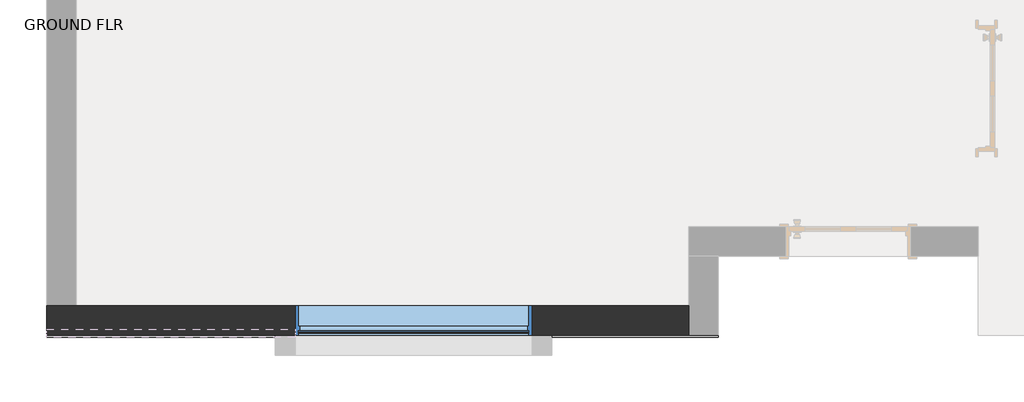
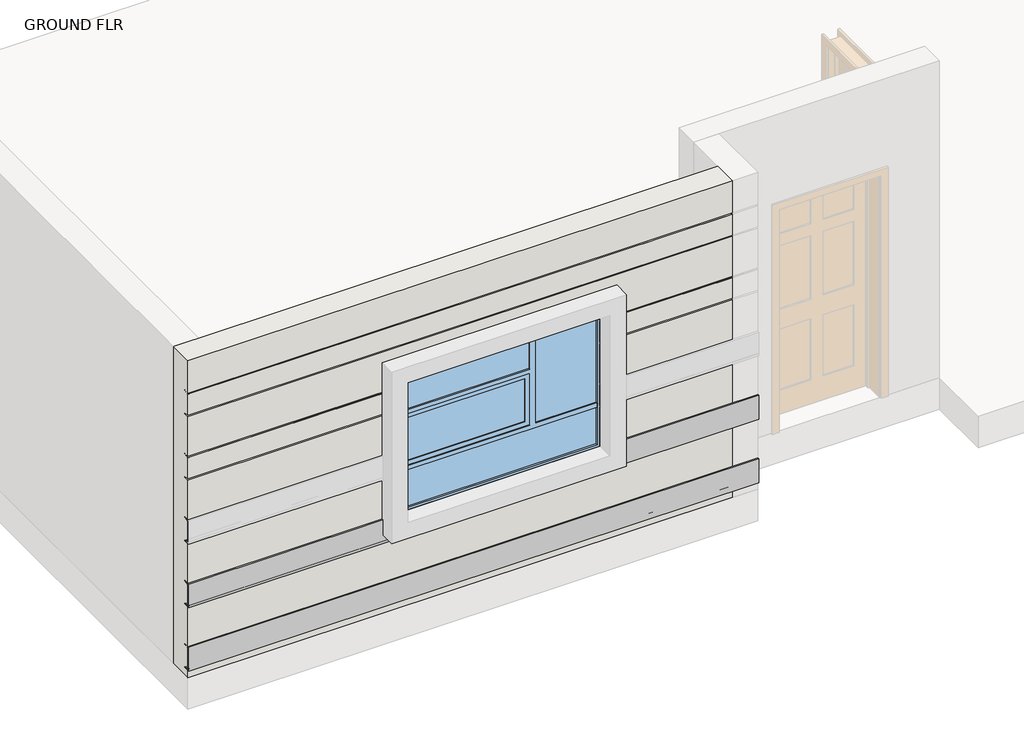
# One storey, part 1 of 4: 2 proxies, 1 wall, 1 window.
"""IFC4 building model written with IfcOpenShell, lengths in millimetres."""

from ifc_helpers import new_model, si_unit, point, frame, frame_2d, origin, place, context, project, spatial, polyline, circle_curve, trimmed, segment, composite_curve, outline, extrude, transform, mapped, element, save
from ifc_brep_helpers import plane_surface, cylinder_surface, revolved_surface, advanced_brep
from components import window_dd9b4f56

model = new_model("IFC4")

# Units and contexts
model_context = context("Model", 3, world=origin())
ifc_project = project(units=[si_unit("LENGTHUNIT", "METRE", prefix="MILLI")], contexts=[model_context])

# Site, building, storey
site = spatial("IfcSite", under=ifc_project)
building = spatial("IfcBuilding", under=site)
storey = spatial("IfcBuildingStorey", under=building, Name="GROUND FLR", Elevation=304.8)

# Proxies
placement = place(None, origin())
element("IfcBuildingElementProxy", 1, Name="Reveal", ObjectType="Reveal", at=placement, inside=storey, context=model_context, shape_type="SweptSolid", body=[
    extrude(outline(composite_curve([segment(polyline([(-2464.7620789, 604.913469), (-2401.5160789, 604.913469), (-2401.5160789, 603.5337932)]), True, "CONTINUOUS"), segment(trimmed(circle_curve(frame_2d((-2406.7611789, 603.5337932)), 5.2451), [point((-2401.5160789, 603.5337932))], [point((-2405.8988881, 598.3600587))], False, "CARTESIAN"), True, "CONTINUOUS"), segment(polyline([(-2405.8988881, 598.3600587), (-2429.5195789, 594.423269), (-2448.7574605, 591.216949)]), True, "CONTINUOUS"), segment(trimmed(circle_curve(frame_2d((-2447.0328789, 580.86948)), 10.4902), [point((-2448.7574605, 591.216949))], [point((-2457.5230789, 580.86948))], True, "CARTESIAN"), True, "CONTINUOUS"), segment(polyline([(-2457.5230789, 580.86948), (-2457.5230789, 400.357458)]), True, "CONTINUOUS"), segment(trimmed(circle_curve(frame_2d((-2447.0328789, 400.357458)), 10.4902), [point((-2457.5230789, 400.357458))], [point((-2448.7574605, 390.009989))], True, "CARTESIAN"), True, "CONTINUOUS"), segment(polyline([(-2448.7574605, 390.009989), (-2429.5195789, 386.803669), (-2405.8988881, 382.8668793)]), True, "CONTINUOUS"), segment(trimmed(circle_curve(frame_2d((-2406.7611789, 377.6931449)), 5.2451), [point((-2405.8988881, 382.8668793))], [point((-2401.5160789, 377.6931449))], False, "CARTESIAN"), True, "CONTINUOUS"), segment(polyline([(-2401.5160789, 377.6931449), (-2401.5160789, 376.313469), (-2464.7620789, 376.313469), (-2464.7620789, 604.913469)]), True, "CONTINUOUS")], self_intersect=False)), frame((-5844.0328791, 0.0, 0.0), z_axis=(1.0, 0.0, 0.0), x_axis=(0.0, 1.0, 0.0)), (0.0, 0.0, 1.0), 5181.6),
])
element("IfcBuildingElementProxy", 2, Name="Reveal", ObjectType="Reveal", at=placement, inside=storey, context=model_context, shape_type="SweptSolid", body=[
    extrude(outline(composite_curve([segment(polyline([(-2464.7620789, 1214.513469), (-2401.5160789, 1214.513469), (-2401.5160789, 1213.1337932)]), True, "CONTINUOUS"), segment(trimmed(circle_curve(frame_2d((-2406.7611789, 1213.1337932)), 5.2451), [point((-2401.5160789, 1213.1337932))], [point((-2405.8988881, 1207.9600587))], False, "CARTESIAN"), True, "CONTINUOUS"), segment(polyline([(-2405.8988881, 1207.9600587), (-2429.5195789, 1204.023269), (-2448.7574605, 1200.816949)]), True, "CONTINUOUS"), segment(trimmed(circle_curve(frame_2d((-2447.0328789, 1190.46948)), 10.4902), [point((-2448.7574605, 1200.816949))], [point((-2457.5230789, 1190.46948))], True, "CARTESIAN"), True, "CONTINUOUS"), segment(polyline([(-2457.5230789, 1190.46948), (-2457.5230789, 1009.957458)]), True, "CONTINUOUS"), segment(trimmed(circle_curve(frame_2d((-2447.0328789, 1009.957458)), 10.4902), [point((-2457.5230789, 1009.957458))], [point((-2448.7574605, 999.609989))], True, "CARTESIAN"), True, "CONTINUOUS"), segment(polyline([(-2448.7574605, 999.609989), (-2429.5195789, 996.403669), (-2405.8988881, 992.4668793)]), True, "CONTINUOUS"), segment(trimmed(circle_curve(frame_2d((-2406.7611789, 987.2931449)), 5.2451), [point((-2405.8988881, 992.4668793))], [point((-2401.5160789, 987.2931449))], False, "CARTESIAN"), True, "CONTINUOUS"), segment(polyline([(-2401.5160789, 987.2931449), (-2401.5160789, 985.913469), (-2464.7620789, 985.913469), (-2464.7620789, 1214.513469)]), True, "CONTINUOUS")], self_intersect=False)), frame((-5844.0328791, 0.0, 0.0), z_axis=(1.0, 0.0, 0.0), x_axis=(0.0, 1.0, 0.0)), (0.0, 0.0, 1.0), 5181.6),
])

# Wall
element("IfcWall", 3, ObjectType="OUTER WALL 9\"", at=placement, inside=storey, context=model_context, shape_type="AdvancedBrep", body=[
    advanced_brep(
    [(-891.0328791, -2221.2776789, 304.8), (-5615.4328791, -2221.2776789, 304.8), (-5844.0328791, -2221.2776789, 304.8), (-5844.0328791, -2221.2776789, 3352.8), (-5615.4328791, -2221.2776789, 3352.8), (-891.0328791, -2221.2776789, 3352.8), (-3926.3328791, -2221.2776789, 2565.4), (-3926.3328791, -2221.2776789, 1219.2), (-2097.5328791, -2221.2776789, 1219.2), (-2097.5328791, -2221.2776789, 2565.4), (-5844.0328791, -2449.8776789, 304.8), (-891.0328791, -2449.8776789, 304.8), (-891.0328791, -2449.8776789, 376.313469), (-5844.0328791, -2449.8776789, 376.313469), (-891.0328791, -2449.8776789, 3352.8), (-5844.0328791, -2449.8776789, 3352.8), (-5844.0328791, -2449.8776789, 3043.313469), (-891.0328791, -2449.8776789, 3043.313469), (-2097.5328791, -2449.8776789, 1219.2), (-3926.3328791, -2449.8776789, 1219.2), (-3926.3328791, -2449.8776789, 1595.513469), (-5844.0328791, -2449.8776789, 1595.513469), (-5844.0328791, -2449.8776789, 1214.513469), (-891.0328791, -2449.8776789, 1214.513469), (-891.0328791, -2449.8776789, 1595.513469), (-2097.5328791, -2449.8776789, 1595.513469), (-3926.3328791, -2449.8776789, 2565.4), (-2097.5328791, -2449.8776789, 2565.4), (-2097.5328791, -2449.8776789, 2433.713469), (-891.0328791, -2449.8776789, 2433.713469), (-891.0328791, -2449.8776789, 2814.713469), (-5844.0328791, -2449.8776789, 2814.713469), (-5844.0328791, -2449.8776789, 2433.713469), (-3926.3328791, -2449.8776789, 2433.713469), (-891.0328791, -2449.8776789, 590.9665791), (-5844.0328791, -2449.8776789, 590.9665791), (-5844.0328791, -2449.8776789, 390.260359), (-891.0328791, -2449.8776789, 390.260359), (-5844.0328791, -2449.8776789, 604.913469), (-891.0328791, -2449.8776789, 604.913469), (-891.0328791, -2449.8776789, 985.913469), (-5844.0328791, -2449.8776789, 985.913469), (-5844.0328791, -2449.8776789, 1200.5665791), (-5844.0328791, -2449.8776789, 999.860359), (-891.0328791, -2449.8776789, 999.860359), (-891.0328791, -2449.8776789, 1200.5665791), (-5844.0328791, -2449.8776789, 3029.3665791), (-5844.0328791, -2449.8776789, 2828.660359), (-891.0328791, -2449.8776789, 2828.660359), (-891.0328791, -2449.8776789, 3029.3665791), (-3926.3328791, -2449.8776789, 2219.060359), (-3926.3328791, -2449.8776789, 2419.7665791), (-5844.0328791, -2449.8776789, 2419.7665791), (-5844.0328791, -2449.8776789, 2219.060359), (-2097.5328791, -2449.8776789, 2419.7665791), (-2097.5328791, -2449.8776789, 2219.060359), (-891.0328791, -2449.8776789, 2219.060359), (-891.0328791, -2449.8776789, 2419.7665791), (-891.0328791, -2449.8776789, 2205.113469), (-2097.5328791, -2449.8776789, 2205.113469), (-2097.5328791, -2449.8776789, 1824.113469), (-891.0328791, -2449.8776789, 1824.113469), (-3926.3328791, -2449.8776789, 2205.113469), (-5844.0328791, -2449.8776789, 2205.113469), (-5844.0328791, -2449.8776789, 1824.113469), (-3926.3328791, -2449.8776789, 1824.113469), (-3926.3328791, -2449.8776789, 1609.460359), (-3926.3328791, -2449.8776789, 1810.1665791), (-5844.0328791, -2449.8776789, 1810.1665791), (-5844.0328791, -2449.8776789, 1609.460359), (-891.0328791, -2449.8776789, 1609.460359), (-891.0328791, -2449.8776789, 1810.1665791), (-2097.5328791, -2449.8776789, 1810.1665791), (-2097.5328791, -2449.8776789, 1609.460359), (-891.0328791, -2401.5160789, 3043.313469), (-891.0328791, -2401.5160789, 3041.9337932), (-891.0328791, -2405.8988881, 3036.7600587), (-891.0328791, -2448.7574605, 3029.616949), (-891.0328791, -2448.7574605, 2828.409989), (-891.0328791, -2405.8988881, 2821.2668793), (-891.0328791, -2401.5160789, 2816.0931449), (-891.0328791, -2401.5160789, 2814.713469), (-891.0328791, -2401.5160789, 2433.713469), (-891.0328791, -2401.5160789, 2432.3337932), (-891.0328791, -2405.8988881, 2427.1600587), (-891.0328791, -2448.7574605, 2420.016949), (-891.0328791, -2448.7574605, 2218.809989), (-891.0328791, -2405.8988881, 2211.6668793), (-891.0328791, -2401.5160789, 2206.4931449), (-891.0328791, -2401.5160789, 2205.113469), (-891.0328791, -2401.5160789, 1824.113469), (-891.0328791, -2401.5160789, 1822.7337932), (-891.0328791, -2405.8988881, 1817.5600587), (-891.0328791, -2448.7574605, 1810.416949), (-891.0328791, -2448.7574605, 1609.209989), (-891.0328791, -2405.8988881, 1602.0668793), (-891.0328791, -2401.5160789, 1596.8931449), (-891.0328791, -2401.5160789, 1595.513469), (-891.0328791, -2401.5160789, 1214.513469), (-891.0328791, -2401.5160789, 1213.1337932), (-891.0328791, -2405.8988881, 1207.9600587), (-891.0328791, -2448.7574605, 1200.816949), (-891.0328791, -2448.7574605, 999.609989), (-891.0328791, -2405.8988881, 992.4668793), (-891.0328791, -2401.5160789, 987.2931449), (-891.0328791, -2401.5160789, 985.913469), (-891.0328791, -2401.5160789, 604.913469), (-891.0328791, -2401.5160789, 603.5337932), (-891.0328791, -2405.8988881, 598.3600587), (-891.0328791, -2448.7574605, 591.216949), (-891.0328791, -2448.7574605, 390.009989), (-891.0328791, -2405.8988881, 382.8668793), (-891.0328791, -2401.5160789, 377.6931449), (-891.0328791, -2401.5160789, 376.313469), (-5844.0328791, -2401.5160789, 376.313469), (-5844.0328791, -2401.5160789, 377.6931449), (-5844.0328791, -2405.8988881, 382.8668793), (-5844.0328791, -2448.7574605, 390.009989), (-5844.0328791, -2448.7574605, 591.216949), (-5844.0328791, -2405.8988881, 598.3600587), (-5844.0328791, -2401.5160789, 603.5337932), (-5844.0328791, -2401.5160789, 604.913469), (-5844.0328791, -2401.5160789, 985.913469), (-5844.0328791, -2401.5160789, 987.2931449), (-5844.0328791, -2405.8988881, 992.4668793), (-5844.0328791, -2448.7574605, 999.609989), (-5844.0328791, -2448.7574605, 1200.816949), (-5844.0328791, -2405.8988881, 1207.9600587), (-5844.0328791, -2401.5160789, 1213.1337932), (-5844.0328791, -2401.5160789, 1214.513469), (-5844.0328791, -2401.5160789, 1595.513469), (-5844.0328791, -2401.5160789, 1596.8931449), (-5844.0328791, -2405.8988881, 1602.0668793), (-5844.0328791, -2448.7574605, 1609.209989), (-5844.0328791, -2448.7574605, 1810.416949), (-5844.0328791, -2405.8988881, 1817.5600587), (-5844.0328791, -2401.5160789, 1822.7337932), (-5844.0328791, -2401.5160789, 1824.113469), (-5844.0328791, -2401.5160789, 2205.113469), (-5844.0328791, -2401.5160789, 2206.4931449), (-5844.0328791, -2405.8988881, 2211.6668793), (-5844.0328791, -2448.7574605, 2218.809989), (-5844.0328791, -2448.7574605, 2420.016949), (-5844.0328791, -2405.8988881, 2427.1600587), (-5844.0328791, -2401.5160789, 2432.3337932), (-5844.0328791, -2401.5160789, 2433.713469), (-5844.0328791, -2401.5160789, 2814.713469), (-5844.0328791, -2401.5160789, 2816.0931449), (-5844.0328791, -2405.8988881, 2821.2668793), (-5844.0328791, -2448.7574605, 2828.409989), (-5844.0328791, -2448.7574605, 3029.616949), (-5844.0328791, -2405.8988881, 3036.7600587), (-5844.0328791, -2401.5160789, 3041.9337932), (-5844.0328791, -2401.5160789, 3043.313469), (-3926.3328791, -2401.5160789, 2433.713469), (-3926.3328791, -2401.5160789, 2432.3337932), (-3926.3328791, -2405.8988881, 2427.1600587), (-3926.3328791, -2448.7574605, 2420.016949), (-3926.3328791, -2448.7574605, 2218.809989), (-3926.3328791, -2405.8988881, 2211.6668793), (-3926.3328791, -2401.5160789, 2206.4931449), (-3926.3328791, -2401.5160789, 2205.113469), (-3926.3328791, -2401.5160789, 1824.113469), (-3926.3328791, -2401.5160789, 1822.7337932), (-3926.3328791, -2405.8988881, 1817.5600587), (-3926.3328791, -2448.7574605, 1810.416949), (-3926.3328791, -2448.7574605, 1609.209989), (-3926.3328791, -2405.8988881, 1602.0668793), (-3926.3328791, -2401.5160789, 1596.8931449), (-3926.3328791, -2401.5160789, 1595.513469), (-2097.5328791, -2401.5160789, 1595.513469), (-2097.5328791, -2401.5160789, 1596.8931449), (-2097.5328791, -2405.8988881, 1602.0668793), (-2097.5328791, -2448.7574605, 1609.209989), (-2097.5328791, -2448.7574605, 1810.416949), (-2097.5328791, -2405.8988881, 1817.5600587), (-2097.5328791, -2401.5160789, 1822.7337932), (-2097.5328791, -2401.5160789, 1824.113469), (-2097.5328791, -2401.5160789, 2205.113469), (-2097.5328791, -2401.5160789, 2206.4931449), (-2097.5328791, -2405.8988881, 2211.6668793), (-2097.5328791, -2448.7574605, 2218.809989), (-2097.5328791, -2448.7574605, 2420.016949), (-2097.5328791, -2405.8988881, 2427.1600587), (-2097.5328791, -2401.5160789, 2432.3337932), (-2097.5328791, -2401.5160789, 2433.713469)],
    [
        (0, 1),
        (1, 2),
        (2, 3),
        (3, 4),
        (4, 5),
        (5, 0),
        (6, 7),
        (7, 8),
        (8, 9),
        (9, 6),
        (10, 11),
        (11, 12),
        (12, 13),
        (13, 10),
        (14, 15),
        (15, 16),
        (16, 17),
        (17, 14),
        (18, 19),
        (19, 20),
        (20, 21),
        (21, 22),
        (22, 23),
        (23, 24),
        (24, 25),
        (25, 18),
        (26, 27),
        (27, 28),
        (28, 29),
        (29, 30),
        (30, 31),
        (31, 32),
        (32, 33),
        (33, 26),
        (34, 35),
        (35, 36),
        (36, 37),
        (37, 34),
        (38, 39),
        (39, 40),
        (40, 41),
        (41, 38),
        (42, 43),
        (43, 44),
        (44, 45),
        (45, 42),
        (46, 47),
        (47, 48),
        (48, 49),
        (49, 46),
        (50, 51),
        (51, 52),
        (52, 53),
        (53, 50),
        (54, 55),
        (55, 56),
        (56, 57),
        (57, 54),
        (58, 59),
        (59, 60),
        (60, 61),
        (61, 58),
        (62, 63),
        (63, 64),
        (64, 65),
        (65, 62),
        (66, 67),
        (67, 68),
        (68, 69),
        (69, 66),
        (70, 71),
        (71, 72),
        (72, 73),
        (73, 70),
        (0, 11),
        (10, 2),
        (3, 15),
        (14, 5),
        (17, 74),
        (74, 75),
        (75, 76, circle_curve(frame((-891.0328791, -2406.7611789, 3041.9337932), z_axis=(-1.0, 0.0, 0.0), x_axis=(0.0, 1.0, 0.0)), 5.2451)),
        (76, 77),
        (77, 49, circle_curve(frame((-891.0328791, -2447.0328789, 3019.26948), z_axis=(1.0, 0.0, 0.0), x_axis=(0.0, 1.0, 0.0)), 10.4902)),
        (48, 78, circle_curve(frame((-891.0328791, -2447.0328789, 2838.757458), z_axis=(1.0, 0.0, 0.0), x_axis=(0.0, 1.0, 0.0)), 10.4902)),
        (78, 79),
        (79, 80, circle_curve(frame((-891.0328791, -2406.7611789, 2816.0931449), z_axis=(-1.0, 0.0, 0.0), x_axis=(0.0, 1.0, 0.0)), 5.2451)),
        (80, 81),
        (81, 30),
        (29, 82),
        (82, 83),
        (83, 84, circle_curve(frame((-891.0328791, -2406.7611789, 2432.3337932), z_axis=(-1.0, 0.0, 0.0), x_axis=(0.0, 1.0, 0.0)), 5.2451)),
        (84, 85),
        (85, 57, circle_curve(frame((-891.0328791, -2447.0328789, 2409.66948), z_axis=(1.0, 0.0, 0.0), x_axis=(0.0, 1.0, 0.0)), 10.4902)),
        (56, 86, circle_curve(frame((-891.0328791, -2447.0328789, 2229.157458), z_axis=(1.0, 0.0, 0.0), x_axis=(0.0, 1.0, 0.0)), 10.4902)),
        (86, 87),
        (87, 88, circle_curve(frame((-891.0328791, -2406.7611789, 2206.4931449), z_axis=(-1.0, 0.0, 0.0), x_axis=(0.0, 1.0, 0.0)), 5.2451)),
        (88, 89),
        (89, 58),
        (61, 90),
        (90, 91),
        (91, 92, circle_curve(frame((-891.0328791, -2406.7611789, 1822.7337932), z_axis=(-1.0, 0.0, 0.0), x_axis=(0.0, 1.0, 0.0)), 5.2451)),
        (92, 93),
        (93, 71, circle_curve(frame((-891.0328791, -2447.0328789, 1800.06948), z_axis=(1.0, 0.0, 0.0), x_axis=(0.0, 1.0, 0.0)), 10.4902)),
        (70, 94, circle_curve(frame((-891.0328791, -2447.0328789, 1619.557458), z_axis=(1.0, 0.0, 0.0), x_axis=(0.0, 1.0, 0.0)), 10.4902)),
        (94, 95),
        (95, 96, circle_curve(frame((-891.0328791, -2406.7611789, 1596.8931449), z_axis=(-1.0, 0.0, 0.0), x_axis=(0.0, 1.0, 0.0)), 5.2451)),
        (96, 97),
        (97, 24),
        (23, 98),
        (98, 99),
        (99, 100, circle_curve(frame((-891.0328791, -2406.7611789, 1213.1337932), z_axis=(-1.0, 0.0, 0.0), x_axis=(0.0, 1.0, 0.0)), 5.2451)),
        (100, 101),
        (101, 45, circle_curve(frame((-891.0328791, -2447.0328789, 1190.46948), z_axis=(1.0, 0.0, 0.0), x_axis=(0.0, 1.0, 0.0)), 10.4902)),
        (44, 102, circle_curve(frame((-891.0328791, -2447.0328789, 1009.957458), z_axis=(1.0, 0.0, 0.0), x_axis=(0.0, 1.0, 0.0)), 10.4902)),
        (102, 103),
        (103, 104, circle_curve(frame((-891.0328791, -2406.7611789, 987.2931449), z_axis=(-1.0, 0.0, 0.0), x_axis=(0.0, 1.0, 0.0)), 5.2451)),
        (104, 105),
        (105, 40),
        (39, 106),
        (106, 107),
        (107, 108, circle_curve(frame((-891.0328791, -2406.7611789, 603.5337932), z_axis=(-1.0, 0.0, 0.0), x_axis=(0.0, 1.0, 0.0)), 5.2451)),
        (108, 109),
        (109, 34, circle_curve(frame((-891.0328791, -2447.0328789, 580.86948), z_axis=(1.0, 0.0, 0.0), x_axis=(0.0, 1.0, 0.0)), 10.4902)),
        (37, 110, circle_curve(frame((-891.0328791, -2447.0328789, 400.357458), z_axis=(1.0, 0.0, 0.0), x_axis=(0.0, 1.0, 0.0)), 10.4902)),
        (110, 111),
        (111, 112, circle_curve(frame((-891.0328791, -2406.7611789, 377.6931449), z_axis=(-1.0, 0.0, 0.0), x_axis=(0.0, 1.0, 0.0)), 5.2451)),
        (112, 113),
        (113, 12),
        (13, 114),
        (114, 115),
        (115, 116, circle_curve(frame((-5844.0328791, -2406.7611789, 377.6931449), z_axis=(1.0, 0.0, 0.0), x_axis=(0.0, 1.0, 0.0)), 5.2451)),
        (116, 117),
        (117, 36, circle_curve(frame((-5844.0328791, -2447.0328789, 400.357458), z_axis=(-1.0, 0.0, 0.0), x_axis=(0.0, 1.0, 0.0)), 10.4902)),
        (35, 118, circle_curve(frame((-5844.0328791, -2447.0328789, 580.86948), z_axis=(-1.0, 0.0, 0.0), x_axis=(0.0, 1.0, 0.0)), 10.4902)),
        (118, 119),
        (119, 120, circle_curve(frame((-5844.0328791, -2406.7611789, 603.5337932), z_axis=(1.0, 0.0, 0.0), x_axis=(0.0, 1.0, 0.0)), 5.2451)),
        (120, 121),
        (121, 38),
        (41, 122),
        (122, 123),
        (123, 124, circle_curve(frame((-5844.0328791, -2406.7611789, 987.2931449), z_axis=(1.0, 0.0, 0.0), x_axis=(0.0, 1.0, 0.0)), 5.2451)),
        (124, 125),
        (125, 43, circle_curve(frame((-5844.0328791, -2447.0328789, 1009.957458), z_axis=(-1.0, 0.0, 0.0), x_axis=(0.0, 1.0, 0.0)), 10.4902)),
        (42, 126, circle_curve(frame((-5844.0328791, -2447.0328789, 1190.46948), z_axis=(-1.0, 0.0, 0.0), x_axis=(0.0, 1.0, 0.0)), 10.4902)),
        (126, 127),
        (127, 128, circle_curve(frame((-5844.0328791, -2406.7611789, 1213.1337932), z_axis=(1.0, 0.0, 0.0), x_axis=(0.0, 1.0, 0.0)), 5.2451)),
        (128, 129),
        (129, 22),
        (21, 130),
        (130, 131),
        (131, 132, circle_curve(frame((-5844.0328791, -2406.7611789, 1596.8931449), z_axis=(1.0, 0.0, 0.0), x_axis=(0.0, 1.0, 0.0)), 5.2451)),
        (132, 133),
        (133, 69, circle_curve(frame((-5844.0328791, -2447.0328789, 1619.557458), z_axis=(-1.0, 0.0, 0.0), x_axis=(0.0, 1.0, 0.0)), 10.4902)),
        (68, 134, circle_curve(frame((-5844.0328791, -2447.0328789, 1800.06948), z_axis=(-1.0, 0.0, 0.0), x_axis=(0.0, 1.0, 0.0)), 10.4902)),
        (134, 135),
        (135, 136, circle_curve(frame((-5844.0328791, -2406.7611789, 1822.7337932), z_axis=(1.0, 0.0, 0.0), x_axis=(0.0, 1.0, 0.0)), 5.2451)),
        (136, 137),
        (137, 64),
        (63, 138),
        (138, 139),
        (139, 140, circle_curve(frame((-5844.0328791, -2406.7611789, 2206.4931449), z_axis=(1.0, 0.0, 0.0), x_axis=(0.0, 1.0, 0.0)), 5.2451)),
        (140, 141),
        (141, 53, circle_curve(frame((-5844.0328791, -2447.0328789, 2229.157458), z_axis=(-1.0, 0.0, 0.0), x_axis=(0.0, 1.0, 0.0)), 10.4902)),
        (52, 142, circle_curve(frame((-5844.0328791, -2447.0328789, 2409.66948), z_axis=(-1.0, 0.0, 0.0), x_axis=(0.0, 1.0, 0.0)), 10.4902)),
        (142, 143),
        (143, 144, circle_curve(frame((-5844.0328791, -2406.7611789, 2432.3337932), z_axis=(1.0, 0.0, 0.0), x_axis=(0.0, 1.0, 0.0)), 5.2451)),
        (144, 145),
        (145, 32),
        (31, 146),
        (146, 147),
        (147, 148, circle_curve(frame((-5844.0328791, -2406.7611789, 2816.0931449), z_axis=(1.0, 0.0, 0.0), x_axis=(0.0, 1.0, 0.0)), 5.2451)),
        (148, 149),
        (149, 47, circle_curve(frame((-5844.0328791, -2447.0328789, 2838.757458), z_axis=(-1.0, 0.0, 0.0), x_axis=(0.0, 1.0, 0.0)), 10.4902)),
        (46, 150, circle_curve(frame((-5844.0328791, -2447.0328789, 3019.26948), z_axis=(-1.0, 0.0, 0.0), x_axis=(0.0, 1.0, 0.0)), 10.4902)),
        (150, 151),
        (151, 152, circle_curve(frame((-5844.0328791, -2406.7611789, 3041.9337932), z_axis=(1.0, 0.0, 0.0), x_axis=(0.0, 1.0, 0.0)), 5.2451)),
        (152, 153),
        (153, 16),
        (6, 26),
        (33, 154),
        (154, 155),
        (155, 156, circle_curve(frame((-3926.3328791, -2406.7611789, 2432.3337932), z_axis=(-1.0, 0.0, 0.0), x_axis=(0.0, 1.0, 0.0)), 5.2451)),
        (156, 157),
        (157, 51, circle_curve(frame((-3926.3328791, -2447.0328789, 2409.66948), z_axis=(1.0, 0.0, 0.0), x_axis=(0.0, 1.0, 0.0)), 10.4902)),
        (50, 158, circle_curve(frame((-3926.3328791, -2447.0328789, 2229.157458), z_axis=(1.0, 0.0, 0.0), x_axis=(0.0, 1.0, 0.0)), 10.4902)),
        (158, 159),
        (159, 160, circle_curve(frame((-3926.3328791, -2406.7611789, 2206.4931449), z_axis=(-1.0, 0.0, 0.0), x_axis=(0.0, 1.0, 0.0)), 5.2451)),
        (160, 161),
        (161, 62),
        (65, 162),
        (162, 163),
        (163, 164, circle_curve(frame((-3926.3328791, -2406.7611789, 1822.7337932), z_axis=(-1.0, 0.0, 0.0), x_axis=(0.0, 1.0, 0.0)), 5.2451)),
        (164, 165),
        (165, 67, circle_curve(frame((-3926.3328791, -2447.0328789, 1800.06948), z_axis=(1.0, 0.0, 0.0), x_axis=(0.0, 1.0, 0.0)), 10.4902)),
        (66, 166, circle_curve(frame((-3926.3328791, -2447.0328789, 1619.557458), z_axis=(1.0, 0.0, 0.0), x_axis=(0.0, 1.0, 0.0)), 10.4902)),
        (166, 167),
        (167, 168, circle_curve(frame((-3926.3328791, -2406.7611789, 1596.8931449), z_axis=(-1.0, 0.0, 0.0), x_axis=(0.0, 1.0, 0.0)), 5.2451)),
        (168, 169),
        (169, 20),
        (19, 7),
        (18, 8),
        (25, 170),
        (170, 171),
        (171, 172, circle_curve(frame((-2097.5328791, -2406.7611789, 1596.8931449), z_axis=(1.0, 0.0, 0.0), x_axis=(0.0, 1.0, 0.0)), 5.2451)),
        (172, 173),
        (173, 73, circle_curve(frame((-2097.5328791, -2447.0328789, 1619.557458), z_axis=(-1.0, 0.0, 0.0), x_axis=(0.0, 1.0, 0.0)), 10.4902)),
        (72, 174, circle_curve(frame((-2097.5328791, -2447.0328789, 1800.06948), z_axis=(-1.0, 0.0, 0.0), x_axis=(0.0, 1.0, 0.0)), 10.4902)),
        (174, 175),
        (175, 176, circle_curve(frame((-2097.5328791, -2406.7611789, 1822.7337932), z_axis=(1.0, 0.0, 0.0), x_axis=(0.0, 1.0, 0.0)), 5.2451)),
        (176, 177),
        (177, 60),
        (59, 178),
        (178, 179),
        (179, 180, circle_curve(frame((-2097.5328791, -2406.7611789, 2206.4931449), z_axis=(1.0, 0.0, 0.0), x_axis=(0.0, 1.0, 0.0)), 5.2451)),
        (180, 181),
        (181, 55, circle_curve(frame((-2097.5328791, -2447.0328789, 2229.157458), z_axis=(-1.0, 0.0, 0.0), x_axis=(0.0, 1.0, 0.0)), 10.4902)),
        (54, 182, circle_curve(frame((-2097.5328791, -2447.0328789, 2409.66948), z_axis=(-1.0, 0.0, 0.0), x_axis=(0.0, 1.0, 0.0)), 10.4902)),
        (182, 183),
        (183, 184, circle_curve(frame((-2097.5328791, -2406.7611789, 2432.3337932), z_axis=(1.0, 0.0, 0.0), x_axis=(0.0, 1.0, 0.0)), 5.2451)),
        (184, 185),
        (185, 28),
        (27, 9),
        (109, 118),
        (108, 119),
        (107, 120),
        (106, 121),
        (117, 110),
        (116, 111),
        (115, 112),
        (113, 114),
        (105, 122),
        (104, 123),
        (103, 124),
        (102, 125),
        (101, 126),
        (100, 127),
        (99, 128),
        (98, 129),
        (81, 146),
        (80, 147),
        (79, 148),
        (78, 149),
        (77, 150),
        (76, 151),
        (75, 152),
        (74, 153),
        (89, 178),
        (88, 179),
        (87, 180),
        (86, 181),
        (85, 182),
        (84, 183),
        (83, 184),
        (82, 185),
        (161, 138),
        (160, 139),
        (159, 140),
        (158, 141),
        (157, 142),
        (156, 143),
        (155, 144),
        (154, 145),
        (97, 170),
        (96, 171),
        (95, 172),
        (94, 173),
        (93, 174),
        (92, 175),
        (91, 176),
        (90, 177),
        (169, 130),
        (168, 131),
        (167, 132),
        (166, 133),
        (165, 134),
        (164, 135),
        (163, 136),
        (162, 137),
    ],
    [
        plane_surface(frame((-662.4328791, -2221.2776789, 304.8), z_axis=(0.0, 1.0, 0.0), x_axis=(-1.0, 0.0, 0.0))),
        plane_surface(frame((-662.4328791, -2449.8776789, 304.8), z_axis=(0.0, -1.0, 0.0), x_axis=(1.0, 0.0, 0.0))),
        plane_surface(frame((-776.7328791, -2221.2776789, 304.8), z_axis=(0.0, 0.0, -1.0), x_axis=(0.0, -1.0, 0.0))),
        plane_surface(frame((-5729.7328791, -2221.2776789, 3352.8), z_axis=(0.0, 0.0, 1.0), x_axis=(0.0, -1.0, 0.0))),
        plane_surface(frame((-891.0328791, -1840.2776789, 304.8), z_axis=(1.0, 0.0, 0.0), x_axis=(0.0, -1.0, 0.0))),
        plane_surface(frame((-5844.0328791, -2449.8776789, 304.8), z_axis=(-1.0, 0.0, 0.0), x_axis=(0.0, -1.0, 0.0))),
        plane_surface(frame((-3926.3328791, -2221.2776789, 2565.4), z_axis=(1.0, 0.0, 0.0), x_axis=(0.0, -1.0, 0.0))),
        plane_surface(frame((-3926.3328791, -2221.2776789, 1219.2), z_axis=(0.0, 0.0, 1.0), x_axis=(0.0, -1.0, 0.0))),
        plane_surface(frame((-2097.5328791, -2221.2776789, 1219.2), z_axis=(-1.0, 0.0, 0.0), x_axis=(0.0, -1.0, 0.0))),
        plane_surface(frame((-2097.5328791, -2221.2776789, 2565.4), z_axis=(0.0, 0.0, -1.0), x_axis=(0.0, -1.0, 0.0))),
        cylinder_surface(frame((-662.4328791, -2447.0328789, 580.86948), z_axis=(-1.0, 0.0, 0.0), x_axis=(0.0, 1.0, 0.0)), 10.4902),
        plane_surface(frame((-662.4328791, -2429.5195789, 594.423269), z_axis=(0.0, -0.16439930721687082, 0.9863938705135049), x_axis=(-1.0, 0.0, 0.0))),
        revolved_surface(polyline([(-891.0328791, -2401.5160788999997, 603.5337932), (-5844.0328791, -2401.5160788999997, 603.5337932)]), (-662.4328791, -2406.7611789, 603.5337932), (1.0, 0.0, 0.0)),
        plane_surface(frame((-662.4328791, -2401.5160789, 603.5337932), z_axis=(0.0, -1.0, 0.0), x_axis=(-1.0, 0.0, 0.0))),
        plane_surface(frame((-662.4328791, -2401.5160789, 604.913469), z_axis=(0.0, 0.0, -1.0), x_axis=(-1.0, 0.0, 0.0))),
        cylinder_surface(frame((-662.4328791, -2447.0328789, 400.357458), z_axis=(-1.0, 0.0, 0.0), x_axis=(0.0, 1.0, 0.0)), 10.4902),
        plane_surface(frame((-662.4328791, -2429.5195789, 386.803669), z_axis=(0.0, -0.1643993072168769, -0.9863938705135039), x_axis=(-1.0, 0.0, 0.0))),
        revolved_surface(polyline([(-891.0328791, -2401.5160788999997, 377.6931449), (-5844.0328791, -2401.5160788999997, 377.6931449)]), (-662.4328791, -2406.7611789, 377.6931449), (1.0, 0.0, 0.0)),
        plane_surface(frame((-662.4328791, -2464.7620789, 376.313469), z_axis=(0.0, 0.0, 1.0), x_axis=(-1.0, 0.0, 0.0))),
        plane_surface(frame((-662.4328791, -2401.5160789, 376.313469), z_axis=(0.0, -1.0, 0.0), x_axis=(-1.0, 0.0, 0.0))),
        plane_surface(frame((-662.4328791, -2464.7620789, 985.913469), z_axis=(0.0, 0.0, 1.0), x_axis=(-1.0, 0.0, 0.0))),
        plane_surface(frame((-662.4328791, -2401.5160789, 985.913469), z_axis=(0.0, -1.0, 0.0), x_axis=(-1.0, 0.0, 0.0))),
        revolved_surface(polyline([(-891.0328791, -2401.5160788999997, 987.2931449), (-5844.0328791, -2401.5160788999997, 987.2931449)]), (-662.4328791, -2406.7611789, 987.2931449), (1.0, 0.0, 0.0)),
        plane_surface(frame((-662.4328791, -2429.5195789, 996.403669), z_axis=(0.0, -0.1643993072168769, -0.9863938705135039), x_axis=(-1.0, 0.0, 0.0))),
        cylinder_surface(frame((-662.4328791, -2447.0328789, 1009.957458), z_axis=(-1.0, 0.0, 0.0), x_axis=(0.0, 1.0, 0.0)), 10.4902),
        cylinder_surface(frame((-662.4328791, -2447.0328789, 1190.46948), z_axis=(-1.0, 0.0, 0.0), x_axis=(0.0, 1.0, 0.0)), 10.4902),
        plane_surface(frame((-662.4328791, -2429.5195789, 1204.023269), z_axis=(0.0, -0.16439930721687082, 0.9863938705135049), x_axis=(-1.0, 0.0, 0.0))),
        revolved_surface(polyline([(-891.0328791, -2401.5160788999997, 1213.1337932), (-5844.0328791, -2401.5160788999997, 1213.1337932)]), (-662.4328791, -2406.7611789, 1213.1337932), (1.0, 0.0, 0.0)),
        plane_surface(frame((-662.4328791, -2401.5160789, 1213.1337932), z_axis=(0.0, -1.0, 0.0), x_axis=(-1.0, 0.0, 0.0))),
        plane_surface(frame((-662.4328791, -2401.5160789, 1214.513469), z_axis=(0.0, 0.0, -1.0), x_axis=(-1.0, 0.0, 0.0))),
        plane_surface(frame((-662.4328791, -2464.7620789, 2814.713469), z_axis=(0.0, 0.0, 1.0), x_axis=(-1.0, 0.0, 0.0))),
        plane_surface(frame((-662.4328791, -2401.5160789, 2814.713469), z_axis=(0.0, -1.0, 0.0), x_axis=(-1.0, 0.0, 0.0))),
        revolved_surface(polyline([(-891.0328791, -2401.5160788999997, 2816.0931449), (-5844.0328791, -2401.5160788999997, 2816.0931449)]), (-662.4328791, -2406.7611789, 2816.0931449), (1.0, 0.0, 0.0)),
        plane_surface(frame((-662.4328791, -2429.5195789, 2825.203669), z_axis=(0.0, -0.1643993072168769, -0.9863938705135039), x_axis=(-1.0, 0.0, 0.0))),
        cylinder_surface(frame((-662.4328791, -2447.0328789, 2838.757458), z_axis=(-1.0, 0.0, 0.0), x_axis=(0.0, 1.0, 0.0)), 10.4902),
        cylinder_surface(frame((-662.4328791, -2447.0328789, 3019.26948), z_axis=(-1.0, 0.0, 0.0), x_axis=(0.0, 1.0, 0.0)), 10.4902),
        plane_surface(frame((-662.4328791, -2429.5195789, 3032.823269), z_axis=(0.0, -0.16439930721687082, 0.9863938705135049), x_axis=(-1.0, 0.0, 0.0))),
        revolved_surface(polyline([(-891.0328791, -2401.5160788999997, 3041.9337932), (-5844.0328791, -2401.5160788999997, 3041.9337932)]), (-662.4328791, -2406.7611789, 3041.9337932), (1.0, 0.0, 0.0)),
        plane_surface(frame((-662.4328791, -2401.5160789, 3041.9337932), z_axis=(0.0, -1.0, 0.0), x_axis=(-1.0, 0.0, 0.0))),
        plane_surface(frame((-662.4328791, -2401.5160789, 3043.313469), z_axis=(0.0, 0.0, -1.0), x_axis=(-1.0, 0.0, 0.0))),
        plane_surface(frame((-662.4328791, -2464.7620789, 2205.113469), z_axis=(0.0, 0.0, 1.0), x_axis=(-1.0, 0.0, 0.0))),
        plane_surface(frame((-662.4328791, -2401.5160789, 2205.113469), z_axis=(0.0, -1.0, 0.0), x_axis=(-1.0, 0.0, 0.0))),
        revolved_surface(polyline([(-891.0328791, -2401.5160788999997, 2206.4931449), (-2097.5328791, -2401.5160788999997, 2206.4931449)]), (-662.4328791, -2406.7611789, 2206.4931449), (1.0, 0.0, 0.0)),
        plane_surface(frame((-662.4328791, -2429.5195789, 2215.603669), z_axis=(0.0, -0.1643993072168769, -0.9863938705135039), x_axis=(-1.0, 0.0, 0.0))),
        cylinder_surface(frame((-662.4328791, -2447.0328789, 2229.157458), z_axis=(-1.0, 0.0, 0.0), x_axis=(0.0, 1.0, 0.0)), 10.4902),
        cylinder_surface(frame((-662.4328791, -2447.0328789, 2409.66948), z_axis=(-1.0, 0.0, 0.0), x_axis=(0.0, 1.0, 0.0)), 10.4902),
        plane_surface(frame((-662.4328791, -2429.5195789, 2423.223269), z_axis=(0.0, -0.16439930721687082, 0.9863938705135049), x_axis=(-1.0, 0.0, 0.0))),
        revolved_surface(polyline([(-891.0328791, -2401.5160788999997, 2432.3337932), (-2097.5328791, -2401.5160788999997, 2432.3337932)]), (-662.4328791, -2406.7611789, 2432.3337932), (1.0, 0.0, 0.0)),
        plane_surface(frame((-662.4328791, -2401.5160789, 2432.3337932), z_axis=(0.0, -1.0, 0.0), x_axis=(-1.0, 0.0, 0.0))),
        plane_surface(frame((-662.4328791, -2401.5160789, 2433.713469), z_axis=(0.0, 0.0, -1.0), x_axis=(-1.0, 0.0, 0.0))),
        plane_surface(frame((-3926.3328791, -2464.7620789, 2205.113469), z_axis=(0.0, 0.0, 1.0), x_axis=(-1.0, 0.0, 0.0))),
        plane_surface(frame((-3926.3328791, -2401.5160789, 2205.113469), z_axis=(0.0, -1.0, 0.0), x_axis=(-1.0, 0.0, 0.0))),
        revolved_surface(polyline([(-3926.3328791, -2401.5160788999997, 2206.4931449), (-5844.0328791, -2401.5160788999997, 2206.4931449)]), (-3926.3328791, -2406.7611789, 2206.4931449), (1.0, 0.0, 0.0)),
        plane_surface(frame((-3926.3328791, -2429.5195789, 2215.603669), z_axis=(0.0, -0.1643993072168769, -0.9863938705135039), x_axis=(-1.0, 0.0, 0.0))),
        cylinder_surface(frame((-3926.3328791, -2447.0328789, 2229.157458), z_axis=(-1.0, 0.0, 0.0), x_axis=(0.0, 1.0, 0.0)), 10.4902),
        cylinder_surface(frame((-3926.3328791, -2447.0328789, 2409.66948), z_axis=(-1.0, 0.0, 0.0), x_axis=(0.0, 1.0, 0.0)), 10.4902),
        plane_surface(frame((-3926.3328791, -2429.5195789, 2423.223269), z_axis=(0.0, -0.16439930721687082, 0.9863938705135049), x_axis=(-1.0, 0.0, 0.0))),
        revolved_surface(polyline([(-3926.3328791, -2401.5160788999997, 2432.3337932), (-5844.0328791, -2401.5160788999997, 2432.3337932)]), (-3926.3328791, -2406.7611789, 2432.3337932), (1.0, 0.0, 0.0)),
        plane_surface(frame((-3926.3328791, -2401.5160789, 2432.3337932), z_axis=(0.0, -1.0, 0.0), x_axis=(-1.0, 0.0, 0.0))),
        plane_surface(frame((-3926.3328791, -2401.5160789, 2433.713469), z_axis=(0.0, 0.0, -1.0), x_axis=(-1.0, 0.0, 0.0))),
        plane_surface(frame((-662.4328791, -2464.7620789, 1595.513469), z_axis=(0.0, 0.0, 1.0), x_axis=(-1.0, 0.0, 0.0))),
        plane_surface(frame((-662.4328791, -2401.5160789, 1595.513469), z_axis=(0.0, -1.0, 0.0), x_axis=(-1.0, 0.0, 0.0))),
        revolved_surface(polyline([(-891.0328791, -2401.5160788999997, 1596.8931449), (-2097.5328791, -2401.5160788999997, 1596.8931449)]), (-662.4328791, -2406.7611789, 1596.8931449), (1.0, 0.0, 0.0)),
        plane_surface(frame((-662.4328791, -2429.5195789, 1606.003669), z_axis=(0.0, -0.1643993072168769, -0.9863938705135039), x_axis=(-1.0, 0.0, 0.0))),
        cylinder_surface(frame((-662.4328791, -2447.0328789, 1619.557458), z_axis=(-1.0, 0.0, 0.0), x_axis=(0.0, 1.0, 0.0)), 10.4902),
        cylinder_surface(frame((-662.4328791, -2447.0328789, 1800.06948), z_axis=(-1.0, 0.0, 0.0), x_axis=(0.0, 1.0, 0.0)), 10.4902),
        plane_surface(frame((-662.4328791, -2429.5195789, 1813.623269), z_axis=(0.0, -0.16439930721687082, 0.9863938705135049), x_axis=(-1.0, 0.0, 0.0))),
        revolved_surface(polyline([(-891.0328791, -2401.5160788999997, 1822.7337932), (-2097.5328791, -2401.5160788999997, 1822.7337932)]), (-662.4328791, -2406.7611789, 1822.7337932), (1.0, 0.0, 0.0)),
        plane_surface(frame((-662.4328791, -2401.5160789, 1822.7337932), z_axis=(0.0, -1.0, 0.0), x_axis=(-1.0, 0.0, 0.0))),
        plane_surface(frame((-662.4328791, -2401.5160789, 1824.113469), z_axis=(0.0, 0.0, -1.0), x_axis=(-1.0, 0.0, 0.0))),
        plane_surface(frame((-3926.3328791, -2464.7620789, 1595.513469), z_axis=(0.0, 0.0, 1.0), x_axis=(-1.0, 0.0, 0.0))),
        plane_surface(frame((-3926.3328791, -2401.5160789, 1595.513469), z_axis=(0.0, -1.0, 0.0), x_axis=(-1.0, 0.0, 0.0))),
        revolved_surface(polyline([(-3926.3328791, -2401.5160788999997, 1596.8931449), (-5844.0328791, -2401.5160788999997, 1596.8931449)]), (-3926.3328791, -2406.7611789, 1596.8931449), (1.0, 0.0, 0.0)),
        plane_surface(frame((-3926.3328791, -2429.5195789, 1606.003669), z_axis=(0.0, -0.1643993072168769, -0.9863938705135039), x_axis=(-1.0, 0.0, 0.0))),
        cylinder_surface(frame((-3926.3328791, -2447.0328789, 1619.557458), z_axis=(-1.0, 0.0, 0.0), x_axis=(0.0, 1.0, 0.0)), 10.4902),
        cylinder_surface(frame((-3926.3328791, -2447.0328789, 1800.06948), z_axis=(-1.0, 0.0, 0.0), x_axis=(0.0, 1.0, 0.0)), 10.4902),
        plane_surface(frame((-3926.3328791, -2429.5195789, 1813.623269), z_axis=(0.0, -0.16439930721687082, 0.9863938705135049), x_axis=(-1.0, 0.0, 0.0))),
        revolved_surface(polyline([(-3926.3328791, -2401.5160788999997, 1822.7337932), (-5844.0328791, -2401.5160788999997, 1822.7337932)]), (-3926.3328791, -2406.7611789, 1822.7337932), (1.0, 0.0, 0.0)),
        plane_surface(frame((-3926.3328791, -2401.5160789, 1822.7337932), z_axis=(0.0, -1.0, 0.0), x_axis=(-1.0, 0.0, 0.0))),
        plane_surface(frame((-3926.3328791, -2401.5160789, 1824.113469), z_axis=(0.0, 0.0, -1.0), x_axis=(-1.0, 0.0, 0.0))),
    ],
    [
        (0, [[1, 2, 3, 4, 5, 6], [7, 8, 9, 10]]),
        (1, [[11, 12, 13, 14]]),
        (1, [[15, 16, 17, 18]]),
        (1, [[19, 20, 21, 22, 23, 24, 25, 26]]),
        (1, [[27, 28, 29, 30, 31, 32, 33, 34]]),
        (1, [[35, 36, 37, 38]]),
        (1, [[39, 40, 41, 42]]),
        (1, [[43, 44, 45, 46]]),
        (1, [[47, 48, 49, 50]]),
        (1, [[51, 52, 53, 54]]),
        (1, [[55, 56, 57, 58]]),
        (1, [[59, 60, 61, 62]]),
        (1, [[63, 64, 65, 66]]),
        (1, [[67, 68, 69, 70]]),
        (1, [[71, 72, 73, 74]]),
        (2, [[-2, -1, 75, -11, 76]]),
        (3, [[-5, -4, 77, -15, 78]]),
        (4, [[-6, -78, -18, 79, 80, 81, 82, 83, -49, 84, 85, 86, 87, 88, -30, 89, 90, 91, 92, 93, -57, 94, 95, 96, 97, 98, -62, 99, 100, 101, 102, 103, -71, 104, 105, 106, 107, 108, -24, 109, 110, 111, 112, 113, -45, 114, 115, 116, 117, 118, -40, 119, 120, 121, 122, 123, -38, 124, 125, 126, 127, 128, -12, -75]]),
        (5, [[-3, -76, -14, 129, 130, 131, 132, 133, -36, 134, 135, 136, 137, 138, -42, 139, 140, 141, 142, 143, -43, 144, 145, 146, 147, 148, -22, 149, 150, 151, 152, 153, -69, 154, 155, 156, 157, 158, -64, 159, 160, 161, 162, 163, -53, 164, 165, 166, 167, 168, -32, 169, 170, 171, 172, 173, -47, 174, 175, 176, 177, 178, -16, -77]]),
        (6, [[-7, 179, -34, 180, 181, 182, 183, 184, -51, 185, 186, 187, 188, 189, -66, 190, 191, 192, 193, 194, -67, 195, 196, 197, 198, 199, -20, 200]]),
        (7, [[-8, -200, -19, 201]]),
        (8, [[-9, -201, -26, 202, 203, 204, 205, 206, -73, 207, 208, 209, 210, 211, -60, 212, 213, 214, 215, 216, -55, 217, 218, 219, 220, 221, -28, 222]]),
        (9, [[-10, -222, -27, -179]]),
        (10, [[223, -134, -35, -123]]),
        (11, [[-223, -122, 224, -135]]),
        (12, [[-224, -121, 225, -136]]),
        (13, [[-225, -120, 226, -137]]),
        (14, [[-226, -119, -39, -138]]),
        (15, [[227, -124, -37, -133]]),
        (16, [[-227, -132, 228, -125]]),
        (17, [[-228, -131, 229, -126]]),
        (18, [[230, -129, -13, -128]]),
        (19, [[-229, -130, -230, -127]]),
        (20, [[231, -139, -41, -118]]),
        (21, [[-231, -117, 232, -140]]),
        (22, [[-232, -116, 233, -141]]),
        (23, [[-233, -115, 234, -142]]),
        (24, [[-234, -114, -44, -143]]),
        (25, [[235, -144, -46, -113]]),
        (26, [[-235, -112, 236, -145]]),
        (27, [[-236, -111, 237, -146]]),
        (28, [[-237, -110, 238, -147]]),
        (29, [[-238, -109, -23, -148]]),
        (30, [[239, -169, -31, -88]]),
        (31, [[-239, -87, 240, -170]]),
        (32, [[-240, -86, 241, -171]]),
        (33, [[-241, -85, 242, -172]]),
        (34, [[-242, -84, -48, -173]]),
        (35, [[243, -174, -50, -83]]),
        (36, [[-243, -82, 244, -175]]),
        (37, [[-244, -81, 245, -176]]),
        (38, [[-245, -80, 246, -177]]),
        (39, [[-246, -79, -17, -178]]),
        (40, [[247, -212, -59, -98]]),
        (41, [[-247, -97, 248, -213]]),
        (42, [[-248, -96, 249, -214]]),
        (43, [[-249, -95, 250, -215]]),
        (44, [[-250, -94, -56, -216]]),
        (45, [[251, -217, -58, -93]]),
        (46, [[-251, -92, 252, -218]]),
        (47, [[-252, -91, 253, -219]]),
        (48, [[-253, -90, 254, -220]]),
        (49, [[-254, -89, -29, -221]]),
        (50, [[255, -159, -63, -189]]),
        (51, [[-255, -188, 256, -160]]),
        (52, [[-256, -187, 257, -161]]),
        (53, [[-257, -186, 258, -162]]),
        (54, [[-258, -185, -54, -163]]),
        (55, [[259, -164, -52, -184]]),
        (56, [[-259, -183, 260, -165]]),
        (57, [[-260, -182, 261, -166]]),
        (58, [[-261, -181, 262, -167]]),
        (59, [[-262, -180, -33, -168]]),
        (60, [[263, -202, -25, -108]]),
        (61, [[-263, -107, 264, -203]]),
        (62, [[-264, -106, 265, -204]]),
        (63, [[-265, -105, 266, -205]]),
        (64, [[-266, -104, -74, -206]]),
        (65, [[267, -207, -72, -103]]),
        (66, [[-267, -102, 268, -208]]),
        (67, [[-268, -101, 269, -209]]),
        (68, [[-269, -100, 270, -210]]),
        (69, [[-270, -99, -61, -211]]),
        (70, [[271, -149, -21, -199]]),
        (71, [[-271, -198, 272, -150]]),
        (72, [[-272, -197, 273, -151]]),
        (73, [[-273, -196, 274, -152]]),
        (74, [[-274, -195, -70, -153]]),
        (75, [[275, -154, -68, -194]]),
        (76, [[-275, -193, 276, -155]]),
        (77, [[-276, -192, 277, -156]]),
        (78, [[-277, -191, 278, -157]]),
        (79, [[-278, -190, -65, -158]]),
    ],
),
])

# Window
window_shape = window_dd9b4f56(model_context)
element("IfcWindow", 4, ObjectType="Window-Awning-Variable : 72\" x 53\" 2", at=placement, inside=storey, context=model_context, shape_type="MappedRepresentation", body=[
    mapped(window_shape, transform((-3011.9328791, -2335.5776789, 304.8), x_axis=(-1.0, 0.0, 0.0), y_axis=(0.0, -1.0, 0.0), z_axis=(0.0, 0.0, 1.0))),
])

save(model, "model.ifc")

# Revit data of these elements
# Type "OUTER WALL 9\""
#   Assembly Code = "B2010"
#   Layers, outside or top first: 0' - 9" "OUTER WALL IVORY WHITE" (function 1)
# Type "Window-Awning-Variable : 72\" x 53\" 2"
#   Type Mark = "21"
#   Fire Rating = "0.5h"
#   Assembly Code = "B2020100"
#   Analytic Construction = "Double glazing - domestic"
#   Window Inset [instance default] = 0' - 0 5/8"
#   Wall Thickness [instance default] = 0' - 6"
#   Visual Light Transmittance = 0.81
#   Transom Height Ratio = 0.3
#   Transom Height = 1' - 3.9"
#   Thermal Resistance (R) = 1.8146 (h·ft²·°F)/BTU
#   Solar Heat Gain Coefficient = 0.76
#   Rough Width = 6' - 0 1/2"
#   Rough Height = 4' - 5 1/2"
#   Opening Window Width = 4' - 0"
#   Opening Window Height = 1' - 9.2"
#   Heat Transfer Coefficient (U) = 0.5511 BTU/(h·ft²·°F)
#   Height = 4' - 5"
#   Frame Gap 3 [instance default] = 0' - 1 83/128"
#   Frame Gap 2 [instance default] = 0' - 0 5/8"
#   Frame Gap 1 = 0' - 1 51/128"
#   Fixed Window Width = 2' - 0"
#   Default Sill Height = 3' - 0"
#   Width = 6' - 0"
#   Frame Material = metal black
#   Glass Panel Material = Glass
#   Wall Closure = (empty or 0)
# Element 3 (IfcWall, "OUTER WALL 9\"")
#   Top Offset = 0' - 0"
#   Base Offset = 0' - 0"
#   wall height = 10' - 0"
#   Phase Created = New Construction
#   Base Constraint = GROUND FLR
#   Top Constraint = FIRST FLOOR
#   Materials on its faces: "OUTER WALL IVORY WHITE"
# Element 4 (IfcWindow, "Window-Awning-Variable : 72\" x 53\" 2")
#   Mark = "1"
#   Window Inset = 0' - 0 5/8"
#   Frame Gap 3 = 0' - 1 83/128"
#   Frame Gap 2 = 0' - 0 5/8"
#   Phase Created = New Construction
#   Materials on its faces: "Glass", "metal black"
# Materials
#   "OUTER WALL IVORY WHITE": class "Generic", colour RGB 120 120 120, transparency 0, Cost = 0
#   "metal black": class "Generic", colour RGB 120 120 120, transparency 0, Cost = 0
#   "Glass": class "Glass", colour RGB 0 128 192, transparency 0.75, Description = "Soda Lime Glass", Cost = 0
# Room at (3477.767, -417.878) mm, phase "New Construction", upper level "GROUND FLR", upper offset 10' - 0", lower offset 0' - 0"
#   Number = "1"
#   Name = "bed room"
# Room at (4239.767, 4738.322) mm, phase "New Construction", upper level "GROUND FLR", upper offset 10' - 0", lower offset 0' - 0"
#   Number = "2"
#   Name = "utility"
# Room at (-90.933, 3150.822) mm, phase "New Construction", upper level "GROUND FLR", upper offset 10' - 0", lower offset 0' - 0"
#   Number = "3"
#   Name = "Dining and living room"
